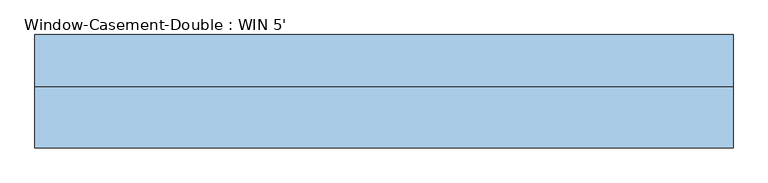
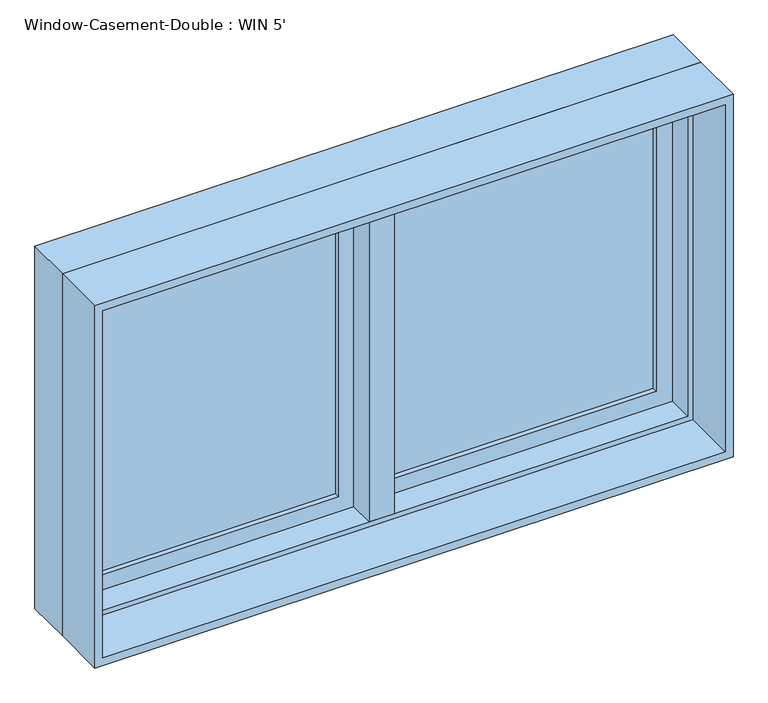
"""IFC4 building model written with IfcOpenShell, lengths in millimetres: window geometry, Window-Casement-Double : WIN 5'."""

from ifc_helpers import new_model, si_unit, frame, origin, place, context, project, spatial, polyline, outline, extrude, faceted_brep, source, transform, mapped, element, save


def window_casement_double_win_5_c1d95f0f(model_context):
    return source(origin(), model_context, "Body", "SolidModel", [
        faceted_brep([(9.525, 133.35, 1816.1), (-9.525, 133.35, 1816.1), (-9.525, 82.55, 1816.1), (9.525, 82.55, 1816.1), (9.525, 133.35, 927.1), (9.525, 82.55, 927.1), (-9.525, 82.55, 927.1), (-9.525, 133.35, 927.1), (-9.525, 82.55, 946.15), (-9.525, 82.55, 1797.05), (-30.1625, 82.55, 946.15), (-30.1625, 82.55, 1797.05), (-30.1625, 19.05, 946.15), (-30.1625, 19.05, 1797.05), (30.1625, 19.05, 946.15), (30.1625, 19.05, 1797.05), (30.1625, 82.55, 946.15), (30.1625, 82.55, 1797.05), (9.525, 82.55, 946.15), (9.525, 82.55, 1797.05)], [[[0, 1, 2, 3]], [[4, 5, 6, 7]], [[1, 0, 4, 7]], [[2, 1, 7, 6, 8, 9]], [[9, 8, 10, 11]], [[11, 10, 12, 13]], [[13, 12, 14, 15]], [[15, 14, 16, 17]], [[17, 16, 18, 19]], [[0, 3, 19, 18, 5, 4]], [[18, 8, 6, 5]], [[9, 19, 3, 2]], [[8, 18, 16, 14, 12, 10]], [[19, 9, 11, 13, 15, 17]]]),
        extrude(outline(polyline([(-66.675, 114.3), (-66.675, 107.95), (-692.15, 107.95), (-692.15, 114.3), (-66.675, 114.3)])), frame((0.0, 0.0, 984.25), z_axis=(0.0, 0.0, 1.0), x_axis=(1.0, 0.0, 0.0)), (0.0, 0.0, 1.0), 774.7),
        extrude(outline(polyline([(-692.15, 95.25), (-692.15, 101.6), (-66.675, 101.6), (-66.675, 95.25), (-692.15, 95.25)])), frame((0.0, 0.0, 984.25), z_axis=(0.0, 0.0, 1.0), x_axis=(1.0, 0.0, 0.0)), (0.0, 0.0, 1.0), 774.7),
        extrude(outline(polyline([(692.15, 114.3), (692.15, 107.95), (66.675, 107.95), (66.675, 114.3), (692.15, 114.3)])), frame((0.0, 0.0, 984.25), z_axis=(0.0, 0.0, 1.0), x_axis=(1.0, 0.0, 0.0)), (0.0, 0.0, 1.0), 774.7),
        extrude(outline(polyline([(66.675, 95.25), (66.675, 101.6), (692.15, 101.6), (692.15, 95.25), (66.675, 95.25)])), frame((0.0, 0.0, 984.25), z_axis=(0.0, 0.0, 1.0), x_axis=(1.0, 0.0, 0.0)), (0.0, 0.0, 1.0), 774.7),
        extrude(outline(polyline([(1816.1, -749.3), (927.1, -749.3), (927.1, -9.525), (1816.1, -9.525), (1816.1, -749.3)]), holes=[polyline([(1758.95, -66.675), (984.25, -66.675), (984.25, -692.15), (1758.95, -692.15), (1758.95, -66.675)])]), frame((0.0, 82.55, 0.0), z_axis=(0.0, 1.0, 0.0), x_axis=(0.0, 0.0, 1.0)), (0.0, 0.0, 1.0), 44.45),
        extrude(outline(polyline([(927.1, 749.3), (1816.1, 749.3), (1816.1, 9.525), (927.1, 9.525), (927.1, 749.3)]), holes=[polyline([(984.25, 66.675), (1758.95, 66.675), (1758.95, 692.15), (984.25, 692.15), (984.25, 66.675)])]), frame((0.0, 82.55, 0.0), z_axis=(0.0, 1.0, 0.0), x_axis=(0.0, 0.0, 1.0)), (0.0, 0.0, 1.0), 44.45),
        extrude(outline(polyline([(1828.8, -762.0), (914.4, -762.0), (914.4, 762.0), (1828.8, 762.0), (1828.8, -762.0)]), holes=[polyline([(1809.75, 742.95), (933.45, 742.95), (933.45, -742.95), (1809.75, -742.95), (1809.75, 742.95)])]), frame((0.0, -114.3, 0.0), z_axis=(0.0, 1.0, 0.0), x_axis=(0.0, 0.0, 1.0)), (0.0, 0.0, 1.0), 133.35),
        faceted_brep([(730.25, 82.55, 1797.05), (730.25, 19.05, 1797.05), (-730.25, 19.05, 1797.05), (-730.25, 82.55, 1797.05), (749.3, 133.35, 1816.1), (749.3, 82.55, 1816.1), (-749.3, 82.55, 1816.1), (-749.3, 133.35, 1816.1), (762.0, 19.05, 1828.8), (762.0, 133.35, 1828.8), (-762.0, 133.35, 1828.8), (-762.0, 19.05, 1828.8), (-730.25, 19.05, 946.15), (-730.25, 82.55, 946.15), (-749.3, 82.55, 927.1), (-749.3, 133.35, 927.1), (-762.0, 133.35, 914.4), (-762.0, 19.05, 914.4), (730.25, 19.05, 946.15), (730.25, 82.55, 946.15), (749.3, 82.55, 927.1), (749.3, 133.35, 927.1), (762.0, 133.35, 914.4), (762.0, 19.05, 914.4)], [[[0, 1, 2, 3]], [[4, 5, 6, 7]], [[8, 9, 10, 11]], [[3, 2, 12, 13]], [[7, 6, 14, 15]], [[11, 10, 16, 17]], [[13, 12, 18, 19]], [[15, 14, 20, 21]], [[17, 16, 22, 23]], [[11, 17, 23, 8], [1, 18, 12, 2]], [[19, 18, 1, 0]], [[5, 20, 14, 6], [3, 13, 19, 0]], [[21, 20, 5, 4]], [[23, 22, 9, 8]], [[9, 22, 16, 10], [7, 15, 21, 4]]]),
    ])


if __name__ == "__main__":
    model = new_model("IFC4")
    model_context = context("Model", 3, world=origin())
    ifc_project = project(units=[si_unit("LENGTHUNIT", "METRE", prefix="MILLI")], contexts=[model_context])
    site = spatial("IfcSite", under=ifc_project)
    building = spatial("IfcBuilding", under=site)
    placement = place(None, origin())
    window_casement_double_win_5_shape = window_casement_double_win_5_c1d95f0f(model_context)
    element("IfcWindow", 1, ObjectType="Window-Casement-Double : WIN 5'", at=placement, inside=building, context=model_context, shape_type="MappedRepresentation", body=[
        mapped(window_casement_double_win_5_shape, transform((0.0, 0.0, 0.0), x_axis=(1.0, 0.0, 0.0), y_axis=(0.0, 1.0, 0.0), z_axis=(0.0, 0.0, 1.0))),
    ])
    save(model, "model.ifc")

# Revit data of these elements
# Type "Window-Casement-Double : WIN 5'"
#   Type Mark = "18"
#   Fire Rating = "0.5h"
#   Assembly Code = "B2020100"
#   Analytic Construction = "Double glazing - domestic"
#   Frame Extension [instance default] = 0' - 0 1/4"
#   Window Inset [instance default] = 0' - 0"
#   Wall Thickness [instance default] = 0' - 6"
#   Interior Wall Closure [instance default] = 0' - 2 1/4"
#   Half Width = 2' - 6"
#   Visual Light Transmittance = 0.81
#   Thermal Resistance (R) = 1.8146 (h·ft²·°F)/BTU
#   Solar Heat Gain Coefficient = 0.76
#   Rough Width = 5' - 0 1/2"
#   Rough Height = 3' - 0 1/2"
#   Height = 3' - 0"
#   Heat Transfer Coefficient (U) = 0.5511 BTU/(h·ft²·°F)
#   Exterior Wall Closure [instance default] = 0' - 1 1/4"
#   Extension Jamb [instance default] = 0' - 2 1/4"
#   Default Sill Height = 3' - 0"
#   Width = 5' - 0"
#   Muntin Visibility = yes
#   Interior Trim Visibility [instance default] = yes
#   Exterior Trim Visibility [instance default] = yes
#   Extension Jamb Visibility [instance default] = yes
#   Interior Trim Material = Wood - Stained
#   Muntin Pattern = Muntin Pattern_2x2 : Muntin Pattern_2x2
#   Interior Trim = Trim-Window-Interior-Flat : Picture Frame
#   Interior Frame Material = Wood - Stained
#   Glass Panel Material = Glass
#   Exterior Trim Material = Clad - White
#   Exterior Trim = Trim-Window-Exterior-Flat : with Sill
#   Exterior Frame Material = Clad - White
#   Wall Closure = (empty or 0)
# Element 1 (IfcWindow, "Window-Casement-Double : WIN 5'")
#   Wall Thickness = 0' - 9"
#   Extension Jamb = 0' - 5 1/4"
#   Materials on its faces: "Wood - Stained", "Glass", "Clad - White"
# Materials
#   "Wood - Stained": class "Wood", colour RGB 224 178 126, transparency 0, Cost = 0
#   "Glass": class "Glass", colour RGB 0 128 192, transparency 0.75, Description = "Soda Lime Glass", Cost = 0
#   "Clad - White": class "Wood", colour RGB 242 242 238, transparency 0, Cost = 0
